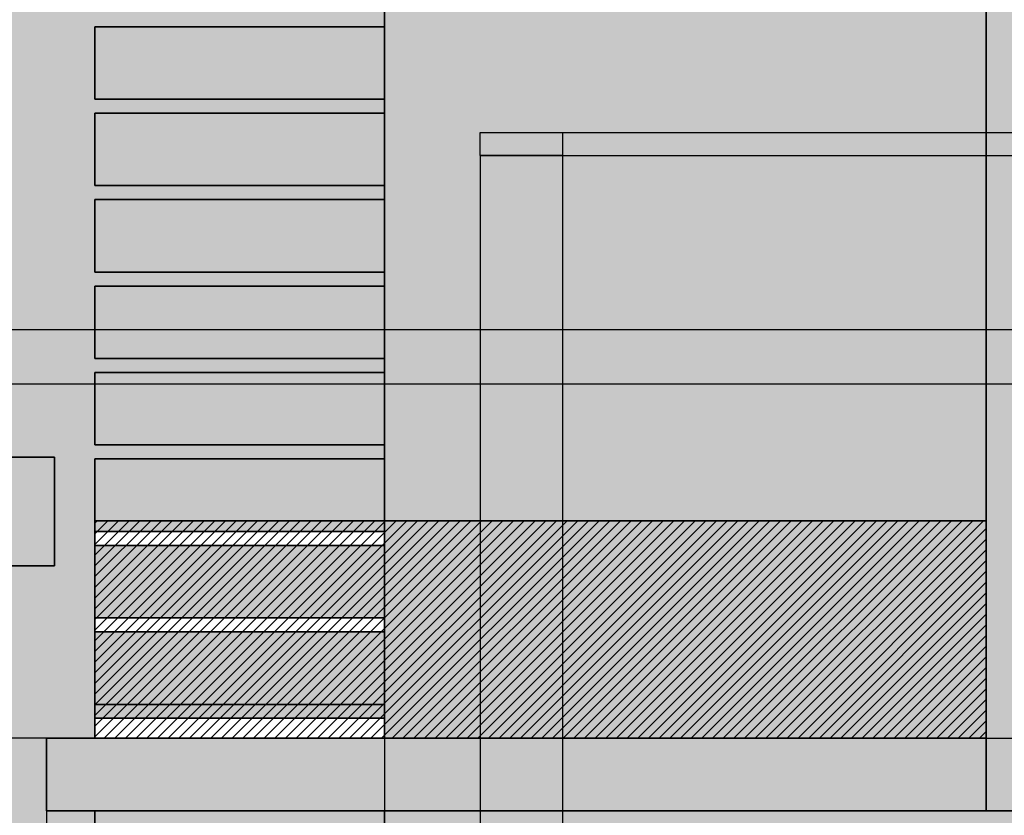
# Model space of a CAD drawing. Units: inches. Extents: x 126 to 726, y 86 to 888.
# Tile 9 of 13: x 426 to 589, y 354 to 486. Entities that reach past the tile are written whole.
import ezdxf

# ---------------------------------------------------------------- set-up
doc = ezdxf.new("R2010")
doc.units = ezdxf.units.IN
doc.header["$MEASUREMENT"] = 0
for name, color, linetype, lineweight in [('A-ANNO-DIMS', 2, 'Continuous', 18), ('A-DOOR', 3, 'Continuous', 25), ('A-ELEV', 7, 'Continuous', 35), ('A-ELEV-PATT', 8, 'Continuous', 13)]:
    doc.layers.add(name, color=color, linetype=linetype, lineweight=lineweight)
doc.styles.get("Standard").update_dxf_attribs({"font": 'arial.ttf'})
doc.dimstyles.get("Standard").update_dxf_attribs({"dimtxt": 6, "dimasz": 3, "dimexe": 0.18, "dimexo": 0.0625, "dimgap": 0.09, "dimtad": 0, "dimtih": 1, "dimtoh": 1, "dimdec": 0, "dimzin": 0, "dimdsep": 46, "dimlunit": 3, "dimtxsty": 'Standard', "dimcen": 0.09, "dimadec": 0, "dimazin": 0, "dimtfac": 1, "dimtdec": 0, "dimtofl": 0, "dimtmove": 0, "dimatfit": 3, "dimfxl": 1, "dimtolj": 1, "dimtzin": 0, "dimarcsym": 0})

# ---------------------------------------------------------------- blocks, each defined once
blk = doc.blocks.new('FACADE-STRIP')
for p, q in [((0, 0), (0, 12)), ((0, 12), (48, 12)), ((0, 0), (48, 0))]:
    blk.add_line(p, q)
blk = doc.blocks.new('*D13')
at = {"layer": 'A-ANNO-DIMS', "color": 0, "lineweight": -2, "transparency": 16777216}
for p, q in [((665.97, 642.98), (665.97, 90.21)), ((185.97, 126.98), (185.97, 90.21)), ((188.97, 90.39), (419.15, 90.39)), ((662.97, 90.39), (432.8, 90.39))]:
    blk.add_line(p, q, dxfattribs=at)
at = {"layer": 'A-ANNO-DIMS', "color": 0, "transparency": 16777216}
for points in [[(188.97, 90.89), (188.97, 89.89), (185.97, 90.39)], [(662.97, 90.89), (662.97, 89.89), (665.97, 90.39)]]:
    blk.add_solid(points, dxfattribs=at)
at = {"layer": 'Defpoints', "color": 0, "transparency": 16777216}
for p in [(665.97, 643.04), (185.97, 127.04), (665.97, 90.39)]:
    blk.add_point(p, dxfattribs=at)
at = {"layer": 'A-ANNO-DIMS', "color": 0, "transparency": 16777216, "insert": (425.97, 90.39), "char_height": 6, "attachment_point": 5}
blk.add_mtext('\\A1;480', dxfattribs=at)
blk = doc.blocks.new('*D18')
at = {"layer": 'A-ANNO-DIMS', "color": 0, "lineweight": -2, "transparency": 16777216}
for p, q in [((431.28, 395.58), (149.14, 395.58)), ((149.32, 392.58), (149.32, 264.47)), ((149.32, 130.04), (149.32, 258.16)), ((185.91, 127.04), (149.14, 127.04))]:
    blk.add_line(p, q, dxfattribs=at)
at = {"layer": 'A-ANNO-DIMS', "color": 0, "transparency": 16777216}
for points in [[(148.82, 392.58), (149.82, 392.58), (149.32, 395.58)], [(148.82, 130.04), (149.82, 130.04), (149.32, 127.04)]]:
    blk.add_solid(points, dxfattribs=at)
at = {"layer": 'Defpoints', "color": 0, "transparency": 16777216}
for p in [(149.32, 395.58), (431.34, 395.58), (185.97, 127.04)]:
    blk.add_point(p, dxfattribs=at)
at = {"layer": 'A-ANNO-DIMS', "color": 0, "transparency": 16777216, "insert": (149.32, 261.31), "char_height": 6, "attachment_point": 5}
blk.add_mtext('\\A1;268.54', dxfattribs=at)
blk = doc.blocks.new('*D19')
at = {"layer": 'A-ANNO-DIMS', "color": 0, "lineweight": -2, "transparency": 16777216}
for p, q in [((233.91, 413.58), (149.14, 413.58)), ((149.32, 410.58), (149.32, 407.74)), ((149.32, 398.58), (149.32, 401.43)), ((431.28, 395.58), (149.14, 395.58))]:
    blk.add_line(p, q, dxfattribs=at)
at = {"layer": 'A-ANNO-DIMS', "color": 0, "transparency": 16777216}
for points in [[(148.82, 410.58), (149.82, 410.58), (149.32, 413.58)], [(148.82, 398.58), (149.82, 398.58), (149.32, 395.58)]]:
    blk.add_solid(points, dxfattribs=at)
at = {"layer": 'Defpoints', "color": 0, "transparency": 16777216}
for p in [(149.32, 413.58), (233.97, 413.58), (431.34, 395.58)]:
    blk.add_point(p, dxfattribs=at)
at = {"layer": 'A-ANNO-DIMS', "color": 0, "transparency": 16777216, "insert": (149.32, 404.58), "char_height": 6, "attachment_point": 5}
blk.add_mtext('\\A1;18', dxfattribs=at)
blk = doc.blocks.new('*D34')
at = {"layer": 'A-ANNO-DIMS', "color": 0, "lineweight": -2, "transparency": 16777216}
for p, q in [((362.73, 524.68), (702.8, 524.68)), ((702.62, 521.68), (702.62, 482.84)), ((702.62, 437.68), (702.62, 476.53)), ((362.73, 434.68), (702.8, 434.68))]:
    blk.add_line(p, q, dxfattribs=at)
at = {"layer": 'A-ANNO-DIMS', "color": 0, "transparency": 16777216}
for points in [[(702.12, 521.68), (703.12, 521.68), (702.62, 524.68)], [(702.12, 437.68), (703.12, 437.68), (702.62, 434.68)]]:
    blk.add_solid(points, dxfattribs=at)
at = {"layer": 'Defpoints', "color": 0, "transparency": 16777216}
for p in [(362.67, 524.68), (702.62, 524.68), (362.67, 434.68)]:
    blk.add_point(p, dxfattribs=at)
at = {"layer": 'A-ANNO-DIMS', "color": 0, "transparency": 16777216, "insert": (702.62, 479.68), "char_height": 6, "attachment_point": 5}
blk.add_mtext('\\A1;90', dxfattribs=at)
blk = doc.blocks.new('*D35')
at = {"layer": 'A-ANNO-DIMS', "color": 0, "lineweight": -2, "transparency": 16777216}
for p, q in [((702.624909, 437.684516), (702.624909, 440.684516)), ((362.728342, 434.684516), (702.804909, 434.684516)), ((371.728342, 425.684516), (702.804909, 425.684516)), ((702.624909, 422.684516), (702.624909, 419.684516))]:
    blk.add_line(p, q, dxfattribs=at)
at = {"layer": 'A-ANNO-DIMS', "color": 0, "transparency": 16777216}
for points in [[(702.124909, 437.684516), (703.124909, 437.684516), (702.624909, 434.684516)], [(702.124909, 422.684516), (703.124909, 422.684516), (702.624909, 425.684516)]]:
    blk.add_solid(points, dxfattribs=at)
at = {"layer": 'Defpoints', "color": 0, "transparency": 16777216}
for p in [(362.665842, 434.684516), (702.624909, 434.684516), (371.665842, 425.684516)]:
    blk.add_point(p, dxfattribs=at)
at = {"layer": 'A-ANNO-DIMS', "color": 0, "transparency": 16777216, "insert": (702.624909, 430.184516), "char_height": 6, "attachment_point": 5}
blk.add_mtext('\\A1;9', dxfattribs=at)
blk = doc.blocks.new('*D42')
at = {"layer": 'A-ANNO-DIMS', "color": 0, "lineweight": -2, "transparency": 16777216}
for p, q in [((429.97, 354.98), (429.97, 90.21)), ((665.97, 354.98), (665.97, 90.21)), ((432.97, 90.39), (541.21, 90.39)), ((662.97, 90.39), (554.74, 90.39))]:
    blk.add_line(p, q, dxfattribs=at)
at = {"layer": 'A-ANNO-DIMS', "color": 0, "transparency": 16777216}
for points in [[(432.97, 90.89), (432.97, 89.89), (429.97, 90.39)], [(662.97, 90.89), (662.97, 89.89), (665.97, 90.39)]]:
    blk.add_solid(points, dxfattribs=at)
at = {"layer": 'Defpoints', "color": 0, "transparency": 16777216}
for p in [(429.97, 355.04), (665.97, 355.04), (665.97, 90.39)]:
    blk.add_point(p, dxfattribs=at)
at = {"layer": 'A-ANNO-DIMS', "color": 0, "transparency": 16777216, "insert": (547.97, 90.39), "char_height": 6, "attachment_point": 5}
blk.add_mtext('\\A1;236', dxfattribs=at)
blk = doc.blocks.new('*D58')
at = {"layer": 'A-ANNO-DIMS', "color": 0, "lineweight": -2, "transparency": 16777216}
for p, q in [((485.91, 533.68), (149.14, 533.68)), ((149.32, 530.68), (149.32, 453.52)), ((149.32, 370.04), (149.32, 447.21)), ((485.91, 367.04), (149.14, 367.04))]:
    blk.add_line(p, q, dxfattribs=at)
at = {"layer": 'A-ANNO-DIMS', "color": 0, "transparency": 16777216}
for points in [[(148.82, 530.68), (149.82, 530.68), (149.32, 533.68)], [(148.82, 370.04), (149.82, 370.04), (149.32, 367.04)]]:
    blk.add_solid(points, dxfattribs=at)
at = {"layer": 'Defpoints', "color": 0, "transparency": 16777216}
for p in [(149.32, 533.68), (485.97, 533.68), (485.97, 367.04)]:
    blk.add_point(p, dxfattribs=at)
at = {"layer": 'A-ANNO-DIMS', "color": 0, "transparency": 16777216, "insert": (149.32, 450.36), "char_height": 6, "attachment_point": 5}
blk.add_mtext('\\A1;166.64', dxfattribs=at)
blk = doc.blocks.new('*D61')
at = {"layer": 'A-ANNO-DIMS', "color": 0, "lineweight": -2, "transparency": 16777216}
for p, q in [((501.82, 463.42), (501.82, 90.21)), ((515.44, 463.42), (515.44, 90.21)), ((504.82, 90.39), (512.44, 90.39)), ((515.44, 90.39), (518.44, 90.39))]:
    blk.add_line(p, q, dxfattribs=at)
at = {"layer": 'A-ANNO-DIMS', "color": 0, "transparency": 16777216}
for points in [[(504.82, 90.89), (504.82, 89.89), (501.82, 90.39)], [(512.44, 90.89), (512.44, 89.89), (515.44, 90.39)]]:
    blk.add_solid(points, dxfattribs=at)
at = {"layer": 'Defpoints', "color": 0, "transparency": 16777216}
for p in [(501.82, 463.48), (515.44, 463.48), (515.44, 90.39)]:
    blk.add_point(p, dxfattribs=at)
at = {"layer": 'A-ANNO-DIMS', "color": 0, "transparency": 16777216, "insert": (530.69, 90.39), "char_height": 6, "attachment_point": 5}
blk.add_mtext('\\A1;13.624', dxfattribs=at)
blk = doc.blocks.new('*D62')
at = {"layer": 'A-ANNO-DIMS', "color": 0, "lineweight": -2, "transparency": 16777216}
for p, q in [((702.62, 470.32), (702.62, 473.32)), ((702.62, 473.32), (705.62, 473.32)), ((515.5, 467.32), (702.8, 467.32)), ((515.5, 463.48), (702.8, 463.48)), ((702.62, 460.48), (702.62, 457.48))]:
    blk.add_line(p, q, dxfattribs=at)
at = {"layer": 'A-ANNO-DIMS', "color": 0, "transparency": 16777216}
for points in [[(702.12, 470.32), (703.12, 470.32), (702.62, 467.32)], [(702.12, 460.48), (703.12, 460.48), (702.62, 463.48)]]:
    blk.add_solid(points, dxfattribs=at)
at = {"layer": 'Defpoints', "color": 0, "transparency": 16777216}
for p in [(515.44, 467.32), (702.62, 467.32), (515.44, 463.48)]:
    blk.add_point(p, dxfattribs=at)
at = {"layer": 'A-ANNO-DIMS', "color": 0, "transparency": 16777216, "insert": (715.84, 473.32), "char_height": 6, "attachment_point": 5}
blk.add_mtext('\\A1;3.839', dxfattribs=at)
blk = doc.blocks.new('*D63')
at = {"layer": 'A-ANNO-DIMS', "color": 0, "lineweight": -2, "transparency": 16777216}
for p, q in [((501.82, 463.42), (501.82, 90.21)), ((485.97, 458.45), (485.97, 90.21)), ((488.97, 90.39), (498.82, 90.39)), ((501.82, 90.39), (504.82, 90.39))]:
    blk.add_line(p, q, dxfattribs=at)
at = {"layer": 'A-ANNO-DIMS', "color": 0, "transparency": 16777216}
for points in [[(488.97, 90.89), (488.97, 89.89), (485.97, 90.39)], [(498.82, 90.89), (498.82, 89.89), (501.82, 90.39)]]:
    blk.add_solid(points, dxfattribs=at)
at = {"layer": 'Defpoints', "color": 0, "transparency": 16777216}
for p in [(501.82, 463.48), (485.97, 458.51), (501.82, 90.39)]:
    blk.add_point(p, dxfattribs=at)
at = {"layer": 'A-ANNO-DIMS', "color": 0, "transparency": 16777216, "insert": (514.74, 90.39), "char_height": 6, "attachment_point": 5}
blk.add_mtext('\\A1;15.84', dxfattribs=at)
blk = doc.blocks.new('*D64')
at = {"layer": 'A-ANNO-DIMS', "color": 0, "lineweight": -2, "transparency": 16777216}
for p, q in [((501.88, 463.48), (702.8, 463.48)), ((702.62, 460.48), (702.62, 418.42)), ((702.62, 370.04), (702.62, 412.11)), ((486.04, 367.04), (702.8, 367.04))]:
    blk.add_line(p, q, dxfattribs=at)
at = {"layer": 'A-ANNO-DIMS', "color": 0, "transparency": 16777216}
for points in [[(702.12, 460.48), (703.12, 460.48), (702.62, 463.48)], [(702.12, 370.04), (703.12, 370.04), (702.62, 367.04)]]:
    blk.add_solid(points, dxfattribs=at)
at = {"layer": 'Defpoints', "color": 0, "transparency": 16777216}
for p in [(501.82, 463.48), (485.97, 367.04), (702.62, 367.04)]:
    blk.add_point(p, dxfattribs=at)
at = {"layer": 'A-ANNO-DIMS', "color": 0, "transparency": 16777216, "insert": (702.62, 415.26), "char_height": 6, "attachment_point": 5}
blk.add_mtext('\\A1;96.44', dxfattribs=at)

msp = doc.modelspace()

# ---------------------------------------------------------------- hatches: boundary and pattern name
at = {"layer": 'A-ELEV-PATT'}
h = msp.add_hatch(color=256, dxfattribs=at)
h.dxf.hatch_style = 1
h.paths.add_polyline_path([(233.9749, 545.5846), (431.3386, 545.5846), (431.3386, 563.5846), (185.9749, 563.5846), (185.9749, 395.5846), (431.3386, 395.5846), (431.3386, 413.5846), (233.9749, 413.5846)])
h.paths.add_polyline_path([(233.9749, 835.0424), (485.9749, 835.0424), (605.9749, 835.0424), (605.9749, 847.0424), (485.9749, 847.0424), (185.9749, 847.0424), (185.9749, 606.5846), (233.9749, 606.5846)])
h.paths.add_polyline_path([(233.9749, 597.5846), (185.9749, 597.5846), (185.9749, 585.5846), (233.9749, 585.5846)])
h.paths.add_polyline_path([(233.9749, 580.5846), (185.9749, 580.5846), (185.9749, 568.5846), (233.9749, 568.5846)])
h = msp.add_hatch(color=256, dxfattribs=at)
h.dxf.hatch_style = 1
h.paths.add_polyline_path([(437.9749, 499.1312), (485.9749, 499.1312), (485.9749, 501.4423), (437.9749, 501.4423), (437.9749, 513.4423), (485.9749, 513.4423), (485.9749, 515.7534), (437.9749, 515.7534), (437.9749, 527.7534), (485.9749, 527.7534), (485.9749, 530.0646), (437.9749, 530.0646), (437.9749, 542.0646), (485.9749, 542.0646), (485.9749, 544.3757), (437.9749, 544.3757), (437.9749, 556.3757), (485.9749, 556.3757), (485.9749, 558.6868), (437.9749, 558.6868), (437.9749, 570.6868), (485.9749, 570.6868), (485.9749, 572.9979), (437.9749, 572.9979), (437.9749, 584.9979), (485.9749, 584.9979), (485.9749, 587.309), (437.9749, 587.309), (437.9749, 595.0424), (429.9749, 595.0424), (429.9749, 607.0424), (437.9749, 607.0424), (437.9749, 615.9312), (437.9749, 630.2423), (437.9749, 642.2423), (485.9749, 642.2423), (485.9749, 644.5534), (437.9749, 644.5534), (437.9749, 656.5534), (485.9749, 656.5534), (485.9749, 658.8645), (437.9749, 658.8645), (437.9749, 670.8645), (485.9749, 670.8645), (485.9749, 673.1757), (437.9749, 673.1757), (437.9749, 685.1757), (485.9749, 685.1757), (485.9749, 687.4868), (437.9749, 687.4868), (437.9749, 699.4868), (485.9749, 699.4868), (485.9749, 701.7979), (437.9749, 701.7979), (437.9749, 713.7979), (485.9749, 713.7979), (485.9749, 716.109), (437.9749, 716.109), (437.9749, 728.109), (485.9749, 728.109), (485.9749, 730.4201), (437.9749, 730.4201), (437.9749, 742.4201), (485.9749, 742.4201), (485.9749, 744.7312), (437.9749, 744.7312), (437.9749, 756.7312), (485.9749, 756.7312), (485.9749, 759.0423), (437.9749, 759.0423), (437.9749, 771.0423), (485.9749, 771.0423), (485.9749, 773.3534), (437.9749, 773.3534), (437.9749, 785.3534), (485.9749, 785.3534), (485.9749, 787.6645), (437.9749, 787.6645), (437.9749, 799.6645), (485.9749, 799.6645), (485.9749, 801.9756), (437.9749, 801.9756), (437.9749, 811.2868), (485.9749, 811.2868), (485.9749, 813.9756), (437.9749, 813.9756), (437.9749, 825.9756), (485.9749, 825.9756), (485.9749, 835.0424), (233.9749, 835.0424), (233.9749, 606.5846), (185.9749, 606.5846), (185.9749, 597.5846), (233.9749, 597.5846), (233.9749, 585.5846), (185.9749, 585.5846), (185.9749, 580.5846), (233.9749, 580.5846), (233.9749, 568.5846), (185.9749, 568.5846), (185.9749, 563.5846), (431.3386, 563.5846), (431.3386, 545.5846), (233.9749, 545.5846), (233.9749, 413.5846), (431.3386, 413.5846), (431.3386, 395.5846), (185.9749, 395.5846), (185.9749, 386.5846), (233.9749, 386.5846), (233.9749, 374.5846), (185.9749, 374.5846), (185.9749, 369.5846), (233.9749, 369.5846), (233.9749, 357.5846), (185.9749, 357.5846), (185.9749, 352.5846), (233.9749, 352.5846), (233.9749, 340.5846), (185.9749, 340.5846), (185.9749, 331.5846), (233.9749, 331.5846), (233.9749, 127.0424), (485.9749, 127.0424), (485.9749, 129.3535), (437.9749, 129.3535), (437.9749, 141.3535), (485.9749, 141.3535), (485.9749, 143.6646), (437.9749, 143.6646), (437.9749, 155.6646), (485.9749, 155.6646), (485.9749, 157.9757), (437.9749, 157.9757), (437.9749, 169.9757), (485.9749, 169.9757), (485.9749, 172.2868), (437.9749, 172.2868), (437.9749, 184.2868), (485.9749, 184.2868), (485.9749, 186.5979), (437.9749, 186.5979), (437.9749, 198.5979), (485.9749, 198.5979), (485.9749, 200.909), (437.9749, 200.909), (437.9749, 212.909), (485.9749, 212.909), (485.9749, 215.2201), (437.9749, 215.2201), (437.9749, 227.2201), (485.9749, 227.2201), (485.9749, 229.5312), (437.9749, 229.5312), (437.9749, 241.5312), (485.9749, 241.5312), (485.9749, 243.8424), (437.9749, 243.8424), (437.9749, 255.8424), (485.9749, 255.8424), (485.9749, 258.1535), (437.9749, 258.1535), (437.9749, 270.1535), (485.9749, 270.1535), (485.9749, 272.4646), (437.9749, 272.4646), (437.9749, 284.4646), (485.9749, 284.4646), (485.9749, 286.7757), (437.9749, 286.7757), (437.9749, 298.7757), (485.9749, 298.7757), (485.9749, 301.0868), (437.9749, 301.0868), (437.9749, 313.0868), (485.9749, 313.0868), (485.9749, 315.3979), (437.9749, 315.3979), (437.9749, 327.3979), (485.9749, 327.3979), (485.9749, 329.709), (437.9749, 329.709), (437.9749, 341.709), (485.9749, 341.709), (485.9749, 344.0201), (437.9749, 344.0201), (437.9749, 355.0424), (429.9749, 355.0424), (429.9749, 367.0424), (437.9749, 367.0424), (437.9749, 372.6423), (437.9749, 386.9535), (437.9749, 401.2646), (437.9749, 413.2646), (485.9749, 413.2646), (485.9749, 415.5757), (437.9749, 415.5757), (437.9749, 427.5757), (485.9749, 427.5757), (485.9749, 429.8868), (437.9749, 429.8868), (437.9749, 441.8868), (485.9749, 441.8868), (485.9749, 444.1979), (437.9749, 444.1979), (437.9749, 456.1979), (485.9749, 456.1979), (485.9749, 458.509), (437.9749, 458.509), (437.9749, 470.509), (485.9749, 470.509), (485.9749, 472.8201), (437.9749, 472.8201), (437.9749, 484.8201), (485.9749, 484.8201), (485.9749, 487.1312), (437.9749, 487.1312)])
h.paths.add_polyline_path([(299.6658, 533.6845), (371.6658, 533.6845), (371.6658, 425.6845), (299.6658, 425.6845)], flags=16)
h.paths.add_polyline_path([(308.6658, 524.6845), (362.6658, 524.6845), (362.6658, 434.6845), (308.6658, 434.6845)], flags=0)
h.paths.add_polyline_path([(317.7956, 603.3211, -0.4129833), (306.8418, 614.321, -0.94403766), (328.769, 615.5845, -0.04423165), (330.7031, 615.4048, -0.89973713), (352.5798, 615.6161, -0.4129833), (363.5336, 604.6162, -0.94403766), (341.6064, 603.3528, -0.04423165), (339.6723, 603.5324, -0.89973713)], flags=16)
h.paths.add_polyline_path([(319.7228, 604.5846, -0.02633223), (319.7726, 605.5306, -0.47905713), (308.8418, 614.321, -1), (326.8418, 614.321, -0.02633223), (326.7919, 613.375, -0.17413188), (332.826, 612.5948, -0.04918553), (332.6526, 614.3527, -1), (350.6526, 614.3527, -0.02633223), (350.6028, 613.4067, -0.47905713), (361.5336, 604.6162, -1), (343.5336, 604.6162, -0.02633223), (343.5834, 605.5622, -0.17413188), (337.5494, 606.3424, -0.04918553), (337.7228, 604.5846, -1)], flags=0)
h.paths.add_polyline_path([(328.769, 355.6561, -0.04423165), (330.7031, 355.4765, -0.89973713), (352.5798, 355.6878, -0.4129833), (363.5336, 344.6879, -0.94403766), (341.6064, 343.4244, -0.04423165), (339.6723, 343.604, -0.89973713), (317.7956, 343.3927, -0.4129833), (306.8418, 354.3926, -0.94403766)], flags=16)
h.paths.add_polyline_path([(326.8418, 354.3926, -0.02633223), (326.7919, 353.4466, -0.17413188), (332.826, 352.6664, -0.04918553), (332.6526, 354.4243, -1), (350.6526, 354.4243, -0.02633223), (350.6028, 353.4783, -0.47905713), (361.5336, 344.6879, -1), (343.5336, 344.6879, -0.02633223), (343.5834, 345.6339, -0.17413188), (337.5494, 346.4141, -0.04918553), (337.7228, 344.6562, -1), (319.7228, 344.6562, -0.02633223), (319.7726, 345.6022, -0.47905713), (308.8418, 354.3926, -1)], flags=0)
h.paths.add_polyline_path([(299.3189, 655.3527), (299.3189, 763.3527), (371.3189, 763.3527), (371.3189, 655.3527)], flags=16)
h.paths.add_polyline_path([(308.3189, 664.3527), (308.3189, 754.3527), (362.3189, 754.3527), (362.3189, 664.3527)], flags=0)
h.paths.add_polyline_path([(299.6658, 303.5875), (371.6658, 303.5875), (371.6658, 195.5875), (299.6658, 195.5875)], flags=16)
h.paths.add_polyline_path([(308.6658, 294.5875), (362.6658, 294.5875), (362.6658, 204.5875), (308.6658, 204.5875)], flags=0)
h.paths.add_polyline_path([(326.3038, 177.3867), (346.055, 177.3867, -0.41421356), (349.055, 174.3867), (349.055, 171.2378), (363.489, 171.2378, -0.41421356), (366.489, 168.2378), (366.489, 159.7133, -0.41421356), (363.489, 156.7133), (343.7379, 156.7133, -0.41421356), (340.7379, 159.7133), (340.7379, 162.8622), (330.5504, 162.8622), (330.5504, 159.7133, -0.41421356), (327.5504, 156.7133), (307.7992, 156.7133, -0.41421356), (304.7992, 159.7133), (304.7992, 168.2378, -0.41421356), (307.7992, 171.2378), (323.3038, 171.2378), (323.3038, 174.3867, -0.41421356)], flags=16)
h.paths.add_polyline_path([(326.3038, 175.3867), (346.055, 175.3867, -0.41421356), (347.055, 174.3867), (347.055, 169.2378), (363.489, 169.2378, -0.41421356), (364.489, 168.2378), (364.489, 159.7133, -0.41421356), (363.489, 158.7133), (343.7379, 158.7133, -0.41421356), (342.7379, 159.7133), (342.7379, 164.8622), (328.5504, 164.8622), (328.5504, 159.7133, -0.41421356), (327.5504, 158.7133), (307.7992, 158.7133, -0.41421356), (306.7992, 159.7133), (306.7992, 168.2378, -0.41421356), (307.7992, 169.2378), (325.3038, 169.2378), (325.3038, 174.3867, -0.41421356)], flags=0)
h = msp.add_hatch(dxfattribs=at)
h.set_pattern_fill('GRAVEL', color=256, scale=40)
h.paths.add_polyline_path([(437.9749, 642.2423), (485.9749, 642.2423), (485.9749, 644.5534), (437.9749, 644.5534), (437.9749, 656.5534), (485.9749, 656.5534), (485.9749, 658.8645), (437.9749, 658.8645), (437.9749, 670.8645), (485.9749, 670.8645), (485.9749, 673.1757), (437.9749, 673.1757), (437.9749, 685.1757), (485.9749, 685.1757), (485.9749, 687.4868), (437.9749, 687.4868), (437.9749, 699.4868), (485.9749, 699.4868), (485.9749, 701.7979), (437.9749, 701.7979), (437.9749, 713.7979), (485.9749, 713.7979), (485.9749, 716.109), (437.9749, 716.109), (437.9749, 728.109), (485.9749, 728.109), (485.9749, 730.4201), (437.9749, 730.4201), (437.9749, 742.4201), (485.9749, 742.4201), (485.9749, 744.7312), (437.9749, 744.7312), (437.9749, 756.7312), (485.9749, 756.7312), (485.9749, 759.0423), (437.9749, 759.0423), (437.9749, 771.0423), (485.9749, 771.0423), (485.9749, 773.3534), (437.9749, 773.3534), (437.9749, 785.3534), (485.9749, 785.3534), (485.9749, 787.6645), (437.9749, 787.6645), (437.9749, 799.6645), (485.9749, 799.6645), (485.9749, 801.9756), (437.9749, 801.9756), (437.9749, 811.2868), (485.9749, 811.2868), (485.9749, 813.9756), (437.9749, 813.9756), (437.9749, 825.9756), (485.9749, 825.9756), (485.9749, 835.0424), (233.9749, 835.0424), (233.9749, 606.5846), (185.9749, 606.5846), (185.9749, 597.5846), (233.9749, 597.5846), (233.9749, 585.5846), (185.9749, 585.5846), (185.9749, 580.5846), (233.9749, 580.5846), (233.9749, 568.5846), (185.9749, 568.5846), (185.9749, 563.5846), (431.3386, 563.5846), (431.3386, 545.5846), (233.9749, 545.5846), (233.9749, 413.5846), (431.3386, 413.5846), (431.3386, 395.5846), (185.9749, 395.5846), (185.9749, 386.5846), (233.9749, 386.5846), (233.9749, 374.5846), (185.9749, 374.5846), (185.9749, 369.5846), (233.9749, 369.5846), (233.9749, 357.5846), (185.9749, 357.5846), (185.9749, 352.5846), (233.9749, 352.5846), (233.9749, 340.5846), (185.9749, 340.5846), (185.9749, 331.5846), (233.9749, 331.5846), (233.9749, 127.0424), (485.9749, 127.0424), (485.9749, 129.3535), (437.9749, 129.3535), (437.9749, 141.3535), (485.9749, 141.3535), (485.9749, 143.6646), (437.9749, 143.6646), (437.9749, 155.6646), (485.9749, 155.6646), (485.9749, 157.9757), (437.9749, 157.9757), (437.9749, 169.9757), (485.9749, 169.9757), (485.9749, 172.2868), (437.9749, 172.2868), (437.9749, 184.2868), (485.9749, 184.2868), (485.9749, 186.5979), (437.9749, 186.5979), (437.9749, 198.5979), (485.9749, 198.5979), (485.9749, 200.909), (437.9749, 200.909), (437.9749, 212.909), (485.9749, 212.909), (485.9749, 215.2201), (437.9749, 215.2201), (437.9749, 227.2201), (485.9749, 227.2201), (485.9749, 229.5312), (437.9749, 229.5312), (437.9749, 241.5312), (485.9749, 241.5312), (485.9749, 243.8424), (437.9749, 243.8424), (437.9749, 255.8424), (485.9749, 255.8424), (485.9749, 258.1535), (437.9749, 258.1535), (437.9749, 270.1535), (485.9749, 270.1535), (485.9749, 272.4646), (437.9749, 272.4646), (437.9749, 284.4646), (485.9749, 284.4646), (485.9749, 286.7757), (437.9749, 286.7757), (437.9749, 298.7757), (485.9749, 298.7757), (485.9749, 301.0868), (437.9749, 301.0868), (437.9749, 313.0868), (485.9749, 313.0868), (485.9749, 315.3979), (437.9749, 315.3979), (437.9749, 327.3979), (485.9749, 327.3979), (485.9749, 329.709), (437.9749, 329.709), (437.9749, 341.709), (485.9749, 341.709), (485.9749, 344.0201), (437.9749, 344.0201), (437.9749, 355.0424), (429.9749, 355.0424), (429.9749, 367.0424), (437.9749, 367.0424), (437.9749, 372.6423), (437.9749, 386.9535), (437.9749, 401.2646), (437.9749, 413.2646), (485.9749, 413.2646), (485.9749, 415.5757), (437.9749, 415.5757), (437.9749, 427.5757), (485.9749, 427.5757), (485.9749, 429.8868), (437.9749, 429.8868), (437.9749, 441.8868), (485.9749, 441.8868), (485.9749, 444.1979), (437.9749, 444.1979), (437.9749, 456.1979), (485.9749, 456.1979), (485.9749, 458.509), (437.9749, 458.509), (437.9749, 470.509), (485.9749, 470.509), (485.9749, 472.8201), (437.9749, 472.8201), (437.9749, 484.8201), (485.9749, 484.8201), (485.9749, 487.1312), (437.9749, 487.1312), (437.9749, 499.1312), (485.9749, 499.1312), (485.9749, 501.4423), (437.9749, 501.4423), (437.9749, 513.4423), (485.9749, 513.4423), (485.9749, 515.7534), (437.9749, 515.7534), (437.9749, 527.7534), (485.9749, 527.7534), (485.9749, 530.0646), (437.9749, 530.0646), (437.9749, 542.0646), (485.9749, 542.0646), (485.9749, 544.3757), (437.9749, 544.3757), (437.9749, 556.3757), (485.9749, 556.3757), (485.9749, 558.6868), (437.9749, 558.6868), (437.9749, 570.6868), (485.9749, 570.6868), (485.9749, 572.9979), (437.9749, 572.9979), (437.9749, 584.9979), (485.9749, 584.9979), (485.9749, 587.309), (437.9749, 587.309), (437.9749, 595.0424), (429.9749, 595.0424), (429.9749, 607.0424), (437.9749, 607.0424), (437.9749, 615.9312), (437.9749, 630.2423)])
h.paths.add_polyline_path([(371.3189, 655.3527), (299.3189, 655.3527), (299.3189, 763.3527), (371.3189, 763.3527)], flags=16)
h.paths.add_polyline_path([(363.5336, 604.6162, -0.94403766), (341.6064, 603.3528, -0.04423165), (339.6723, 603.5324, -0.89973713), (317.7956, 603.3211, -0.4129833), (306.8418, 614.321, -0.94403766), (328.769, 615.5845, -0.04423165), (330.7031, 615.4048, -0.89973713), (352.5798, 615.6161, -0.4129833)], flags=16)
h.paths.add_polyline_path([(361.5336, 604.6162, -1), (343.5336, 604.6162, -0.02633223), (343.5834, 605.5622, -0.17413188), (337.5494, 606.3424, -0.04918553), (337.7228, 604.5846, -1), (319.7228, 604.5846, -0.02633223), (319.7726, 605.5306, -0.47905713), (308.8418, 614.321, -1), (326.8418, 614.321, -0.02633223), (326.7919, 613.375, -0.17413188), (332.826, 612.5948, -0.04918553), (332.6526, 614.3527, -1), (350.6526, 614.3527, -0.02633223), (350.6028, 613.4067, -0.47905713)], flags=0)
h.paths.add_polyline_path([(362.3189, 664.3527), (308.3189, 664.3527), (308.3189, 754.3527), (362.3189, 754.3527)], flags=0)
h.paths.add_polyline_path([(371.6658, 533.6845), (371.6658, 425.6845), (299.6658, 425.6845), (299.6658, 533.6845)], flags=16)
h.paths.add_polyline_path([(362.6658, 524.6845), (362.6658, 434.6845), (308.6658, 434.6845), (308.6658, 524.6845)], flags=0)
h.paths.add_polyline_path([(352.5798, 355.6878, -0.4129833), (363.5336, 344.6879, -0.94403766), (341.6064, 343.4244, -0.04423165), (339.6723, 343.604, -0.89973713), (317.7956, 343.3927, -0.4129833), (306.8418, 354.3926, -0.94403766), (328.769, 355.6561, -0.04423165), (330.7031, 355.4765, -0.89973713)], flags=16)
h.paths.add_polyline_path([(350.6526, 354.4243, -0.02633223), (350.6028, 353.4783, -0.47905713), (361.5336, 344.6879, -1), (343.5336, 344.6879, -0.02633223), (343.5834, 345.6339, -0.17413188), (337.5494, 346.4141, -0.04918553), (337.7228, 344.6562, -1), (319.7228, 344.6562, -0.02633223), (319.7726, 345.6022, -0.47905713), (308.8418, 354.3926, -1), (326.8418, 354.3926, -0.02633223), (326.7919, 353.4466, -0.17413188), (332.826, 352.6664, -0.04918553), (332.6526, 354.4243, -1)], flags=0)
h.paths.add_polyline_path([(371.6658, 303.5875), (371.6658, 195.5875), (299.6658, 195.5875), (299.6658, 303.5875)], flags=16)
h.paths.add_polyline_path([(362.6658, 294.5875), (362.6658, 204.5875), (308.6658, 204.5875), (308.6658, 294.5875)], flags=0)
h.paths.add_polyline_path([(346.055, 177.3867, -0.41421356), (349.055, 174.3867), (349.055, 171.2378), (363.489, 171.2378, -0.41421356), (366.489, 168.2378), (366.489, 159.7133, -0.41421356), (363.489, 156.7133), (343.7379, 156.7133, -0.41421356), (340.7379, 159.7133), (340.7379, 162.8622), (330.5504, 162.8622), (330.5504, 159.7133, -0.41421356), (327.5504, 156.7133), (307.7992, 156.7133, -0.41421356), (304.7992, 159.7133), (304.7992, 168.2378, -0.41421356), (307.7992, 171.2378), (323.3038, 171.2378), (323.3038, 174.3867, -0.41421356), (326.3038, 177.3867)], flags=16)
h.paths.add_polyline_path([(346.055, 175.3867, -0.41421356), (347.055, 174.3867), (347.055, 169.2378), (363.489, 169.2378, -0.41421356), (364.489, 168.2378), (364.489, 159.7133, -0.41421356), (363.489, 158.7133), (343.7379, 158.7133, -0.41421356), (342.7379, 159.7133), (342.7379, 164.8622), (328.5504, 164.8622), (328.5504, 159.7133, -0.41421356), (327.5504, 158.7133), (307.7992, 158.7133, -0.41421356), (306.7992, 159.7133), (306.7992, 168.2378, -0.41421356), (307.7992, 169.2378), (325.3038, 169.2378), (325.3038, 174.3867, -0.41421356), (326.3038, 175.3867)], flags=0)
h = msp.add_hatch(color=256, dxfattribs=at)
h.dxf.hatch_style = 1
h.paths.add_polyline_path([(485.9749, 427.5757), (437.9749, 427.5757), (437.9749, 415.5757), (485.9749, 415.5757)])
h.paths.add_polyline_path([(485.9749, 441.8868), (437.9749, 441.8868), (437.9749, 429.8868), (485.9749, 429.8868)])
h.paths.add_polyline_path([(485.9749, 456.1979), (437.9749, 456.1979), (437.9749, 444.1979), (485.9749, 444.1979)])
h.paths.add_polyline_path([(485.9749, 470.509), (437.9749, 470.509), (437.9749, 458.509), (485.9749, 458.509)])
h.paths.add_polyline_path([(485.9749, 484.8201), (437.9749, 484.8201), (437.9749, 472.8201), (485.9749, 472.8201)])
h.paths.add_polyline_path([(485.9749, 499.1312), (437.9749, 499.1312), (437.9749, 487.1312), (485.9749, 487.1312)])
h.paths.add_polyline_path([(485.9749, 513.4423), (437.9749, 513.4423), (437.9749, 501.4423), (485.9749, 501.4423)])
h.paths.add_polyline_path([(485.9749, 527.7534), (437.9749, 527.7534), (437.9749, 515.7534), (485.9749, 515.7534)])
h.paths.add_polyline_path([(485.9749, 542.0646), (437.9749, 542.0646), (437.9749, 530.0646), (485.9749, 530.0646)])
h.paths.add_polyline_path([(485.9749, 556.3757), (437.9749, 556.3757), (437.9749, 544.3757), (485.9749, 544.3757)])
h.paths.add_polyline_path([(485.9749, 570.6868), (437.9749, 570.6868), (437.9749, 558.6868), (485.9749, 558.6868)])
h.paths.add_polyline_path([(485.9749, 584.9979), (437.9749, 584.9979), (437.9749, 572.9979), (485.9749, 572.9979)])
h.paths.add_polyline_path([(485.9749, 595.0424), (437.9749, 595.0424), (437.9749, 587.309), (485.9749, 587.309)])
h.paths.add_polyline_path([(485.9749, 613.6201), (437.9749, 613.6201), (437.9749, 607.0424), (485.9749, 607.0424)])
h.paths.add_polyline_path([(485.9749, 627.9312), (437.9749, 627.9312), (437.9749, 615.9312), (485.9749, 615.9312)])
h.paths.add_polyline_path([(485.9749, 642.2423), (437.9749, 642.2423), (437.9749, 630.2423), (485.9749, 630.2423)])
h.paths.add_polyline_path([(485.9749, 656.5534), (437.9749, 656.5534), (437.9749, 644.5534), (485.9749, 644.5534)])
h.paths.add_polyline_path([(485.9749, 670.8645), (437.9749, 670.8645), (437.9749, 658.8645), (485.9749, 658.8645)])
h.paths.add_polyline_path([(485.9749, 685.1757), (437.9749, 685.1757), (437.9749, 673.1757), (485.9749, 673.1757)])
h.paths.add_polyline_path([(485.9749, 699.4868), (437.9749, 699.4868), (437.9749, 687.4868), (485.9749, 687.4868)])
h.paths.add_polyline_path([(485.9749, 713.7979), (437.9749, 713.7979), (437.9749, 701.7979), (485.9749, 701.7979)])
h.paths.add_polyline_path([(485.9749, 728.109), (437.9749, 728.109), (437.9749, 716.109), (485.9749, 716.109)])
h.paths.add_polyline_path([(485.9749, 742.4201), (437.9749, 742.4201), (437.9749, 730.4201), (485.9749, 730.4201)])
h.paths.add_polyline_path([(485.9749, 756.7312), (437.9749, 756.7312), (437.9749, 744.7312), (485.9749, 744.7312)])
h.paths.add_polyline_path([(485.9749, 771.0423), (437.9749, 771.0423), (437.9749, 759.0423), (485.9749, 759.0423)])
h.paths.add_polyline_path([(485.9749, 785.3534), (437.9749, 785.3534), (437.9749, 773.3534), (485.9749, 773.3534)])
h.paths.add_polyline_path([(485.9749, 799.6645), (437.9749, 799.6645), (437.9749, 787.6645), (485.9749, 787.6645)])
h.paths.add_polyline_path([(485.9749, 811.2868), (437.9749, 811.2868), (437.9749, 801.9756), (485.9749, 801.9756)])
h.paths.add_polyline_path([(485.9749, 825.9756), (437.9749, 825.9756), (437.9749, 813.9756), (485.9749, 813.9756)])
h = msp.add_hatch(color=256, dxfattribs=at)
h.dxf.hatch_style = 1
h.paths.add_polyline_path([(655.5818, 607.0424), (655.5818, 611.0424), (637.5818, 611.0424), (637.5818, 355.0424), (655.5818, 355.0424)])
h.paths.add_polyline_path([(629.5818, 611.0424), (611.5818, 611.0424), (611.5818, 355.0424), (629.5818, 355.0424)])
h.paths.add_polyline_path([(585.5818, 355.0424), (603.5818, 355.0424), (603.5818, 611.0424), (585.5818, 611.0424), (585.5818, 607.0424)])
h = msp.add_hatch(color=256, dxfattribs=at)
h.dxf.hatch_style = 1
h.paths.add_polyline_path([(437.9749, 367.0424), (429.9749, 367.0424), (429.9749, 355.0424), (437.9749, 355.0424), (585.5818, 355.0424), (585.5818, 367.0424)])
h.paths.add_polyline_path([(585.5818, 595.0424), (585.5818, 607.0424), (437.9749, 607.0424), (429.9749, 607.0424), (429.9749, 595.0424), (437.9749, 595.0424)])
h = msp.add_hatch(color=256, dxfattribs=at)
h.dxf.hatch_style = 1
h.paths.add_polyline_path([(485.9749, 595.0424), (485.9749, 564.6845), (585.5818, 564.6845), (585.5818, 595.0424)])
h.paths.add_polyline_path([(660.0469, 325.0424), (660.0469, 355.0424), (485.9749, 355.0424), (485.9749, 325.0424)])
h = msp.add_hatch(color=256, dxfattribs=at)
h.dxf.hatch_style = 1
h.paths.add_polyline_path([(585.5818, 533.6845), (485.9749, 533.6845), (485.9749, 403.0424), (585.5818, 403.0424)])
h.paths.add_polyline_path([(515.4403, 467.321), (515.4403, 463.4817), (501.8163, 463.4817), (501.8163, 467.321)], flags=16)
h = msp.add_hatch(color=256, dxfattribs=at)
h.dxf.hatch_style = 1
h.paths.add_polyline_path([(515.4403, 260.2201), (501.8163, 260.2201), (501.8163, 256.3808), (515.4403, 256.3808)])
h.paths.add_polyline_path([(515.4403, 467.321), (501.8163, 467.321), (501.8163, 463.4817), (515.4403, 463.4817)])
h = msp.add_hatch(color=256, dxfattribs=at)
h.dxf.hatch_style = 1
h.paths.add_polyline_path([(485.9749, 413.2646), (437.9749, 413.2646), (437.9749, 403.0424), (485.9749, 403.0424)])
h.paths.add_polyline_path([(485.9749, 403.0424), (437.9749, 403.0424), (437.9749, 401.2646), (485.9749, 401.2646)])
h = msp.add_hatch(dxfattribs=at)
h.set_pattern_fill('ANSI31', color=256, scale=10)
h.paths.add_polyline_path([(585.5818, 403.0424), (485.9749, 403.0424), (485.9749, 367.0424), (585.5818, 367.0424)])
h.paths.add_polyline_path([(485.9749, 398.9535), (437.9749, 398.9535), (437.9749, 386.9535), (485.9749, 386.9535)])
h.paths.add_polyline_path([(485.9749, 384.6423), (437.9749, 384.6423), (437.9749, 372.6423), (485.9749, 372.6423)])
h.paths.add_polyline_path([(485.9749, 370.3312), (437.9749, 370.3312), (437.9749, 367.0424), (485.9749, 367.0424)])
h.paths.add_polyline_path([(485.9749, 386.9535), (437.9749, 386.9535), (437.9749, 384.6423), (485.9749, 384.6423)])
h.paths.add_polyline_path([(485.9749, 372.6423), (437.9749, 372.6423), (437.9749, 370.3312), (485.9749, 370.3312)])
h.paths.add_polyline_path([(485.9749, 403.0424), (437.9749, 403.0424), (437.9749, 401.2646), (485.9749, 401.2646)])
h.paths.add_polyline_path([(485.9749, 401.2646), (437.9749, 401.2646), (437.9749, 398.9535), (485.9749, 398.9535)])
h = msp.add_hatch(color=256, dxfattribs=at)
h.dxf.hatch_style = 1
h.paths.add_polyline_path([(585.5818, 403.0424), (485.9749, 403.0424), (485.9749, 367.0424), (585.5818, 367.0424)])
h.paths.add_polyline_path([(527.9749, 235.0424), (519.9749, 235.0424), (519.9749, 133.0424), (527.9749, 133.0424)])
h.paths.add_polyline_path([(513.9749, 235.0424), (505.9749, 235.0424), (505.9749, 133.0424), (513.9749, 133.0424)])
h.paths.add_polyline_path([(499.9749, 235.0424), (491.9749, 235.0424), (491.9749, 133.0424), (499.9749, 133.0424)])
h = msp.add_hatch(color=256, dxfattribs=at)
h.dxf.hatch_style = 1
h.paths.add_polyline_path([(485.9749, 129.3535), (485.9749, 141.3535), (437.9749, 141.3535), (437.9749, 129.3535)])
h.paths.add_polyline_path([(437.9749, 155.6646), (437.9749, 143.6646), (485.9749, 143.6646), (485.9749, 155.6646)])
h.paths.add_polyline_path([(485.9749, 157.9757), (485.9749, 169.9757), (437.9749, 169.9757), (437.9749, 157.9757)])
h.paths.add_polyline_path([(485.9749, 172.2868), (485.9749, 184.2868), (437.9749, 184.2868), (437.9749, 172.2868)])
h.paths.add_polyline_path([(485.9749, 186.5979), (485.9749, 198.5979), (437.9749, 198.5979), (437.9749, 186.5979)])
h.paths.add_polyline_path([(485.9749, 200.909), (485.9749, 212.909), (437.9749, 212.909), (437.9749, 200.909)])
h.paths.add_polyline_path([(485.9749, 215.2201), (485.9749, 227.2201), (437.9749, 227.2201), (437.9749, 215.2201)])
h.paths.add_polyline_path([(437.9749, 241.5312), (437.9749, 229.5312), (485.9749, 229.5312), (485.9749, 241.5312)])
h.paths.add_polyline_path([(485.9749, 243.8424), (485.9749, 255.8424), (437.9749, 255.8424), (437.9749, 243.8424)])
h.paths.add_polyline_path([(485.9749, 258.1535), (485.9749, 270.1535), (437.9749, 270.1535), (437.9749, 258.1535)])
h.paths.add_polyline_path([(485.9749, 272.4646), (485.9749, 284.4646), (437.9749, 284.4646), (437.9749, 272.4646)])
h.paths.add_polyline_path([(485.9749, 286.7757), (485.9749, 298.7757), (437.9749, 298.7757), (437.9749, 286.7757)])
h.paths.add_polyline_path([(437.9749, 313.0868), (437.9749, 301.0868), (485.9749, 301.0868), (485.9749, 313.0868)])
h.paths.add_polyline_path([(437.9749, 327.3979), (437.9749, 315.3979), (485.9749, 315.3979), (485.9749, 327.3979)])
h.paths.add_polyline_path([(485.9749, 329.709), (485.9749, 341.709), (437.9749, 341.709), (437.9749, 329.709)])
h.paths.add_polyline_path([(485.9749, 344.0201), (485.9749, 355.0424), (437.9749, 355.0424), (437.9749, 344.0201)])
h.paths.add_polyline_path([(437.9749, 384.6423), (437.9749, 372.6423), (485.9749, 372.6423), (485.9749, 384.6423)])
h.paths.add_polyline_path([(437.9749, 398.9535), (437.9749, 386.9535), (485.9749, 386.9535), (485.9749, 398.9535)])
h = msp.add_hatch(color=256, dxfattribs=at)
h.dxf.hatch_style = 1
h.paths.add_polyline_path([(485.9749, 372.6423), (437.9749, 372.6423), (437.9749, 370.3312), (485.9749, 370.3312)])

# ---------------------------------------------------------------- linework, layer by layer
at = {"layer": 'A-DOOR'}
msp.add_lwpolyline([(501.8163, 467.321), (515.4403, 467.321), (515.4403, 463.4817), (501.8163, 463.4817)], close=True, dxfattribs=at)
at = {"layer": 'A-ELEV'}
for p, q in [((585.5818, 355.0424), (585.5818, 607.0424)), ((485.9749, 367.0424), (485.9749, 595.0424)), ((431.3386, 413.5846), (233.9749, 413.5846)), ((431.3386, 395.5846), (431.3386, 413.5846)), ((437.9749, 413.2646), (485.9749, 413.2646)), ((437.9749, 401.2646), (437.9749, 413.2646)), ((437.9749, 403.0424), (585.5818, 403.0424)), ((437.9749, 401.2646), (485.9749, 401.2646)), ((437.9749, 386.9535), (437.9749, 401.2646)), ((437.9749, 398.9535), (485.9749, 398.9535)), ((431.3386, 395.5846), (185.9749, 395.5846)), ((437.9749, 386.9535), (485.9749, 386.9535)), ((437.9749, 372.6423), (437.9749, 386.9535)), ((437.9749, 384.6423), (485.9749, 384.6423)), ((437.9749, 372.6423), (485.9749, 372.6423)), ((437.9749, 367.0424), (437.9749, 372.6423)), ((437.9749, 370.3312), (485.9749, 370.3312)), ((429.9749, 355.0424), (429.9749, 367.0424)), ((429.9749, 367.0424), (437.9749, 367.0424)), ((437.9749, 367.0424), (585.5818, 367.0424)), ((437.9749, 355.0424), (429.9749, 355.0424)), ((665.9749, 355.0424), (437.9749, 355.0424)), ((437.9749, 344.0201), (437.9749, 355.0424)), ((485.9749, 127.0424), (485.9749, 355.0424))]:
    msp.add_line(p, q, dxfattribs=at)

# ---------------------------------------------------------------- block references
for p in [(437.975, 472.8196), (437.975, 458.5085), (437.975, 444.1974), (437.975, 429.8863), (437.975, 415.5752)]:
    msp.add_blockref('FACADE-STRIP', p, dxfattribs=at)

# ---------------------------------------------------------------- dimensions: what is measured, and where the dimension line sits
at = {"layer": 'A-ANNO-DIMS'}
for base, p1, p2, override, picture, middle in [((665.9749, 90.3924), (185.9749, 127.0424), (665.9749, 643.0424), {"dimdec": 0, "dimlfac": 1, "dimrnd": 0, "dimzin": 0, "dimdsep": 46, "dimlunit": 2}, '*D13', (425.9749, 90.3924)), ((501.8163, 90.3924), (485.9749, 458.509), (501.8163, 463.4817), {"dimdec": 2, "dimlfac": 1, "dimrnd": 0, "dimzin": 0, "dimdsep": 46, "dimlunit": 2}, '*D63', (514.7351, 90.3924)), ((515.4403, 90.3924), (501.8163, 463.4817), (515.4403, 463.4817), {"dimdec": 3, "dimlfac": 1, "dimrnd": 0, "dimzin": 0, "dimdsep": 46, "dimlunit": 2}, '*D61', (530.6899, 90.3924)), ((665.9749, 90.3924), (429.9749, 355.0424), (665.9749, 355.0424), {"dimdec": 0, "dimlfac": 1, "dimrnd": 0, "dimzin": 0, "dimdsep": 46, "dimlunit": 2}, '*D42', (547.9749, 90.3924))]:
    dim = msp.add_linear_dim(base=base, p1=p1, p2=p2, dimstyle='Standard', override=override, dxfattribs=at)
    dim.commit()
    dim.dimension.update_dxf_attribs({"geometry": picture, "text_midpoint": middle})
for base, p1, p2, override, picture, middle in [((149.3249, 533.6845), (485.9749, 367.0424), (485.9749, 533.6845), {"dimdec": 2, "dimlfac": 1, "dimrnd": 0, "dimzin": 0, "dimdsep": 46, "dimlunit": 2}, '*D58', (149.3249, 450.3634)), ((702.6249, 524.6845), (362.6658, 434.6845), (362.6658, 524.6845), {"dimdec": 0, "dimlfac": 1, "dimrnd": 0, "dimzin": 0, "dimdsep": 46, "dimlunit": 2}, '*D34', (702.6249, 479.6845)), ((702.6249, 467.321), (515.4403, 463.4817), (515.4403, 467.321), {"dimdec": 3, "dimlfac": 1, "dimrnd": 0, "dimzin": 0, "dimdsep": 46, "dimlunit": 2}, '*D62', (715.8425, 473.321)), ((702.6249, 367.0424), (501.8163, 463.4817), (485.9749, 367.0424), {"dimdec": 2, "dimlfac": 1, "dimrnd": 0, "dimzin": 0, "dimdsep": 46, "dimlunit": 2}, '*D64', (702.6249, 415.262)), ((702.6249, 434.6845), (371.6658, 425.6845), (362.6658, 434.6845), {"dimdec": 0, "dimlfac": 1, "dimrnd": 0, "dimzin": 0, "dimdsep": 46, "dimlunit": 2}, '*D35', (702.6249, 430.1845)), ((149.3249, 413.5846), (431.3386, 395.5846), (233.9749, 413.5846), {"dimdec": 0, "dimlfac": 1, "dimrnd": 0, "dimzin": 0, "dimdsep": 46, "dimlunit": 2}, '*D19', (149.3249, 404.5846)), ((149.3249, 395.5846), (185.9749, 127.0424), (431.3386, 395.5846), {"dimdec": 2, "dimlfac": 1, "dimrnd": 0, "dimzin": 0, "dimdsep": 46, "dimlunit": 2}, '*D18', (149.3249, 261.3135))]:
    dim = msp.add_linear_dim(base=base, p1=p1, p2=p2, angle=90, dimstyle='Standard', override=override, dxfattribs=at)
    dim.commit()
    dim.dimension.update_dxf_attribs({"geometry": picture, "text_midpoint": middle})

doc.saveas('drawing.dxf')
